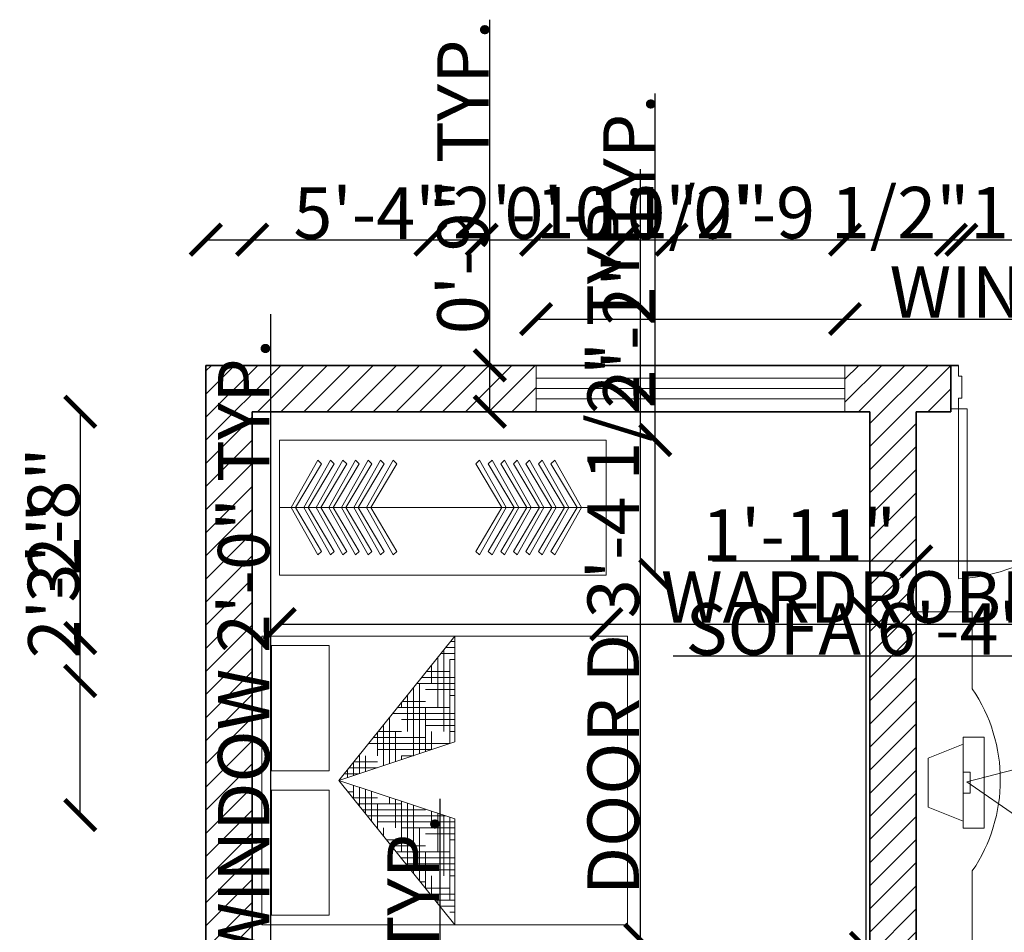
# Model space of a CAD drawing. Units: inches. Extents: x 1957 to 2456, y 1504 to 2088.
# Tile 5 of 6: x 2029 to 2220, y 1911 to 2088. Entities that reach past the tile are written whole.
import ezdxf

# ---------------------------------------------------------------- set-up
doc = ezdxf.new("R2010")
doc.units = ezdxf.units.IN
doc.header["$LTSCALE"] = 2
for name, color, linetype, lineweight in [('A-ANNO-DIMS', 2, 'Continuous', 18), ('A-FURN', 8, 'Continuous', 18), ('A-WALL-PATT', 8, 'Continuous', 13), ('Doors', 42, 'Continuous', 18), ('shelves', 204, 'Continuous', 18), ('Walls', 7, 'Continuous', 35), ('Windows', 140, 'Continuous', 18)]:
    doc.layers.add(name, color=color, linetype=linetype, lineweight=lineweight)
doc.styles.get("Standard").update_dxf_attribs({"font": 'arial.ttf'})
doc.dimstyles.get("Standard").update_dxf_attribs({"dimtxt": 10, "dimasz": 6, "dimexe": 0.18, "dimexo": 0.0625, "dimgap": 0.09, "dimtad": 1, "dimdec": 1, "dimzin": 0, "dimdsep": 46, "dimlunit": 4, "dimtxsty": 'Standard', "dimblk": 'ARCHTICK', "dimcen": 0.09, "dimse1": 1, "dimse2": 1, "dimadec": 0, "dimazin": 0, "dimtfac": 1, "dimtdec": 1, "dimtofl": 0, "dimtmove": 0, "dimatfit": 3, "dimfxl": 1, "dimtolj": 1, "dimtzin": 0, "dimarcsym": 0})

# ---------------------------------------------------------------- blocks, each defined once
blk = doc.blocks.new('banghe81')
for p, q in [((-500, 3000), (0, 3000)), ((-500, 2312.5), (-500, 3000)), ((0, 3000), (0, 0)), ((-606.9, 1930), (-419.4, 1930)), ((-606.9, 1117.5), (-606.9, 1930)), ((-419.4, 1930), (-419.4, 1117.5)), ((-106.9, 1742.5), (-419.4, 1867.5)), ((-924.7, 1843.4), (-449.7, 1516.6)), ((-106.9, 1305), (-106.9, 1742.5)), ((-481.9, 1617.5), (-481.9, 1430)), ((-419.4, 1617.5), (-481.9, 1617.5)), ((-449.7, 1516.6), (-1057.1, 1361)), ((-481.9, 1430), (-419.4, 1430)), ((-419.4, 1180), (-106.9, 1305)), ((-419.4, 1117.5), (-606.9, 1117.5)), ((-500, 0), (-500, 687.5)), ((0, 0), (-500, 0)), ((-500, 0), (-500, 0))]:
    blk.add_line(p, q)
blk.add_arc((695.3, 1500), 1445.3, 145.79454, 214.20546)
blk = doc.blocks.new('*X4')
at = {"color": 0}
for p, q in [((20.25, 14.8125), (20.2772, 14.8125)), ((20.1739, 14.75), (20.2772, 14.75)), ((20.1875, 14.75), (20.1875, 14.7669)), ((20.199, 14.7812), (20.2772, 14.7812)), ((20.25, 14.3194), (20.25, 14.75)), ((20.1236, 14.6875), (20.25, 14.6875)), ((20.125, 14.5), (20.125, 14.6893)), ((20.1487, 14.7188), (20.2772, 14.7188)), ((20.1562, 14.625), (20.1562, 14.7281)), ((20.0938, 14.375), (20.0938, 14.6504)), ((20.0984, 14.6562), (20.125, 14.6562)), ((20.0625, 14.2573), (20.0625, 14.6116)), ((20.125, 14.5938), (20.2772, 14.5938)), ((20.2188, 14.3091), (20.2188, 14.625)), ((20.25, 14.625), (20.2772, 14.625)), ((19.9979, 14.5312), (20.2772, 14.5312)), ((20.023, 14.5625), (20.2772, 14.5625)), ((20.0312, 14.2469), (20.0312, 14.5727)), ((19.9727, 14.5), (20.25, 14.5)), ((20, 14.2366), (20, 14.5)), ((20.1875, 14.2987), (20.1875, 14.5)), ((19.9225, 14.4375), (20, 14.4375)), ((19.9476, 14.4688), (20.125, 14.4688)), ((20.25, 14.4375), (20.2772, 14.4375)), ((19.875, 14.25), (19.875, 14.3785)), ((19.9062, 14.375), (19.9062, 14.4174)), ((19.9688, 14.2262), (19.9688, 14.375)), ((20, 14.375), (20.2772, 14.375)), ((20.125, 14.4062), (20.2772, 14.4062)), ((20.1562, 14.2884), (20.1562, 14.375)), ((19.8438, 14.1848), (19.8438, 14.3397)), ((19.875, 14.3438), (20.2772, 14.3438)), ((19.7967, 14.2812), (20.125, 14.2812)), ((19.8125, 14.1744), (19.8125, 14.3008)), ((19.8219, 14.3125), (20.2291, 14.3125)), ((19.75, 14.1537), (19.75, 14.2231)), ((19.7716, 14.25), (20, 14.25)), ((19.7812, 14.1641), (19.7812, 14.262)), ((19.9375, 14.2159), (19.9375, 14.25)), ((19.7213, 14.1875), (19.75, 14.1875)), ((19.7465, 14.2188), (19.875, 14.2188)), ((19.7018, 14.0938), (19.7786, 14.0938)), ((19.7188, 14.0726), (19.7188, 14.1136)), ((19.75, 14.0338), (19.75, 14.1032)), ((19.7812, 13.9949), (19.7812, 14.0929)), ((19.8125, 14), (19.8125, 14.0825)), ((19.7269, 14.0625), (19.8728, 14.0625)), ((19.752, 14.0312), (19.875, 14.0312)), ((19.9062, 13.8396), (19.9062, 14.0514)), ((19.9375, 13.8007), (19.9375, 14.0411)), ((19.9688, 13.875), (19.9688, 14.0307)), ((20, 14), (20, 14.0204)), ((19.875, 13.8784), (19.875, 14)), ((19.875, 13.9688), (20.1557, 13.9688)), ((20, 14), (20.0614, 14)), ((20.0625, 13.6454), (20.0625, 13.9996)), ((20.0938, 13.625), (20.0938, 13.9893)), ((20.125, 13.75), (20.125, 13.9789)), ((20.1562, 13.875), (20.1562, 13.9686)), ((19.8275, 13.9375), (20.25, 13.9375)), ((20.25, 13.5), (20.25, 13.9375)), ((19.8526, 13.9062), (20.125, 13.9062)), ((19.8777, 13.875), (20, 13.875)), ((20.0312, 13.6842), (20.0312, 13.875)), ((20.2188, 13.4511), (20.2188, 13.875)), ((20.25, 13.875), (20.2772, 13.875)), ((20, 13.8125), (20.2772, 13.8125)), ((20.125, 13.8438), (20.2772, 13.8438)), ((19.9532, 13.7812), (20.2772, 13.7812)), ((19.9783, 13.75), (20.25, 13.75)), ((20, 13.723), (20, 13.75)), ((20.0035, 13.7188), (20.125, 13.7188)), ((20.1875, 13.49), (20.1875, 13.75)), ((20.25, 13.6875), (20.2772, 13.6875)), ((20.0789, 13.625), (20.2772, 13.625)), ((20.125, 13.6562), (20.2772, 13.6562)), ((20.1562, 13.5288), (20.1562, 13.625)), ((20.104, 13.5938), (20.2772, 13.5938)), ((20.1292, 13.5625), (20.25, 13.5625)), ((20.2046, 13.4688), (20.2772, 13.4688)), ((20.25, 13.5), (20.2772, 13.5)), ((20.2297, 13.4375), (20.2772, 13.4375)), ((20.2549, 13.4062), (20.2772, 13.4062))]:
    blk.add_line(p, q, dxfattribs=at)
blk = doc.blocks.new('MAT-P13')
for p, q in [((-0.75, 0), (0.75, 0)), ((-0.75, 0), (-0.75, -1.9)), ((0.75, 0), (0.75, -1.9)), ((-0.7, -0.05), (-0.7, -0.35)), ((-0.7, -0.05), (-0.05, -0.05)), ((-0.05, -0.35), (-0.05, -0.05)), ((0.05, -0.05), (0.7, -0.05)), ((0.05, -0.35), (0.05, -0.05)), ((0.7, -0.05), (0.7, -0.35)), ((-0.7, -0.35), (-0.05, -0.35)), ((0.05, -0.35), (0.7, -0.35)), ((-0.75, -1.0034), (0, -0.4)), ((0, -0.4), (-0.75, -1.0034)), ((0, -0.4), (-0.2, -1.0034)), ((0, -0.4), (0.2, -1.0034)), ((0, -0.4), (0.75, -1.0034)), ((-0.75, -1.0034), (-0.2, -1.0034)), ((0.2, -1.0034), (0.75, -1.0034)), ((0.75, -1.9), (-0.75, -1.9))]:
    blk.add_line(p, q)
at = {"xscale": -1, "rotation": 90}
blk.add_blockref('*X4', (14.1285, 19.2738), dxfattribs=at)
blk = doc.blocks.new('AP0B05')
for p, q in [((35, 100), (35, 880)), ((75, 100), (75, 878.9))]:
    blk.add_line(p, q)
for points in [[(0, 100), (0, -100), (35, -100), (35, -50), (50, -50), (50, 50), (35, 50), (35, 100)], [(850, 100), (850, -100), (815, -100), (815, -50), (800, -50), (800, 50), (815, 50), (815, 100)]]:
    blk.add_lwpolyline(points, close=True)
blk.add_lwpolyline([(35, 100), (75, 100)])
blk.add_arc((-2.4, 62.6), 818.3, 2.6212, 87.3788)
blk = doc.blocks.new('WIN-60IN')
for p, q in [((0, 6.5), (60, 6.5)), ((0, 4.5), (60, 4.5)), ((0, 2.5), (60, 2.5))]:
    blk.add_line(p, q)
blk.add_lwpolyline([(0, 9), (60, 9), (60, 0), (0, 0)], close=True)
blk = doc.blocks.new('WARDROBE-RAIL')
blk.add_line((0, 13.12), (63.46, 13.12))
blk.add_lwpolyline([(0, 26.23), (63.46, 26.23), (63.46, 0), (0, 0)], close=True)
for points in [[(2.25, 13.12), (7.43, 22.31), (8.16, 21.63), (3.1, 13.12)], [(4.68, 13.12), (9.87, 22.31), (10.6, 21.63), (5.54, 13.12)], [(7.12, 13.12), (12.3, 22.31), (13.03, 21.63), (7.98, 13.12)], [(9.56, 13.12), (14.74, 22.31), (15.47, 21.63), (10.41, 13.12)], [(11.99, 13.12), (17.18, 22.31), (17.91, 21.63), (12.85, 13.12)], [(14.43, 13.12), (19.61, 22.31), (20.34, 21.63), (15.29, 13.12)], [(16.87, 13.12), (22.05, 22.31), (22.78, 21.63), (17.72, 13.12)], [(44.01, 13.12), (38.82, 22.31), (38.09, 21.63), (43.15, 13.12)], [(46.44, 13.12), (41.26, 22.31), (40.53, 21.63), (45.59, 13.12)], [(48.88, 13.12), (43.7, 22.31), (42.96, 21.63), (48.02, 13.12)], [(51.31, 13.12), (46.13, 22.31), (45.4, 21.63), (50.46, 13.12)], [(53.75, 13.12), (48.57, 22.31), (47.84, 21.63), (52.89, 13.12)], [(56.19, 13.12), (51.01, 22.31), (50.27, 21.63), (55.33, 13.12)], [(58.62, 13.12), (53.44, 22.31), (52.71, 21.63), (57.77, 13.12)], [(2.25, 13.12), (7.43, 3.92), (8.16, 4.61), (3.1, 13.12)], [(4.68, 13.12), (9.87, 3.92), (10.6, 4.61), (5.54, 13.12)], [(7.12, 13.12), (12.3, 3.92), (13.03, 4.61), (7.98, 13.12)], [(9.56, 13.12), (14.74, 3.92), (15.47, 4.61), (10.41, 13.12)], [(11.99, 13.12), (17.18, 3.92), (17.91, 4.61), (12.85, 13.12)], [(14.43, 13.12), (19.61, 3.92), (20.34, 4.61), (15.29, 13.12)], [(16.87, 13.12), (22.05, 3.92), (22.78, 4.61), (17.72, 13.12)], [(44.01, 13.12), (38.82, 3.92), (38.09, 4.61), (43.15, 13.12)], [(46.44, 13.12), (41.26, 3.92), (40.53, 4.61), (45.59, 13.12)], [(48.88, 13.12), (43.7, 3.92), (42.96, 4.61), (48.02, 13.12)], [(51.31, 13.12), (46.13, 3.92), (45.4, 4.61), (50.46, 13.12)], [(53.75, 13.12), (48.57, 3.92), (47.84, 4.61), (52.89, 13.12)], [(56.19, 13.12), (51.01, 3.92), (50.27, 4.61), (55.33, 13.12)], [(58.62, 13.12), (53.44, 3.92), (52.71, 4.61), (57.77, 13.12)]]:
    blk.add_lwpolyline(points)
blk = doc.blocks.new('_ArchTick')
at = {"color": 0, "linetype": 'ByBlock', "const_width": 0.15}
blk.add_lwpolyline([(-0.5, -0.5), (0.5, 0.5)], dxfattribs=at)
blk = doc.blocks.new('*D17')
at = {"layer": 'A-ANNO-DIMS', "color": 0, "lineweight": -2, "transparency": 16777216}
for p, q in [((2149.43, 1909.65), (2149.43, 2059.35)), ((2149.43, 1869.22), (2149.43, 1909.65))]:
    blk.add_line(p, q, dxfattribs=at)
at = {"layer": 'Defpoints', "color": 0, "transparency": 16777216}
for p in [(2149.43, 1909.65), (2155.49, 1909.65), (2155.49, 1869.22)]:
    blk.add_point(p, dxfattribs=at)
at = {"layer": 'A-ANNO-DIMS', "color": 0, "lineweight": -2, "transparency": 16777216, "xscale": 6, "yscale": 6, "zscale": 6}
for p, rotation in [((2149.43, 1909.65), 90), ((2149.43, 1869.22), 270)]:
    blk.add_blockref('_ArchTick', p, dxfattribs=dict(at, rotation=rotation))
at = {"layer": 'A-ANNO-DIMS', "color": 0, "transparency": 16777216, "insert": (2144.16, 1987.5), "char_height": 10, "attachment_point": 5, "rotation": 90}
blk.add_mtext('\\A1;DOOR D 3\'-4 1/2" TYP.', dxfattribs=at)
blk = doc.blocks.new('*D21')
at = {"layer": 'A-ANNO-DIMS', "color": 0, "lineweight": -2, "transparency": 16777216}
for p, q in [((2110.57, 1795.08), (2110.57, 1937.02)), ((2110.57, 1760.22), (2110.57, 1795.08))]:
    blk.add_line(p, q, dxfattribs=at)
at = {"layer": 'Defpoints', "color": 0, "transparency": 16777216}
for p in [(2110.57, 1795.08), (2115.8, 1795.08), (2115.8, 1760.22)]:
    blk.add_point(p, dxfattribs=at)
at = {"layer": 'A-ANNO-DIMS', "color": 0, "lineweight": -2, "transparency": 16777216, "xscale": 6, "yscale": 6, "zscale": 6}
for p, rotation in [((2110.57, 1795.08), 90), ((2110.57, 1760.22), 270)]:
    blk.add_blockref('_ArchTick', p, dxfattribs=dict(at, rotation=rotation))
at = {"layer": 'A-ANNO-DIMS', "color": 0, "transparency": 16777216, "insert": (2105.3, 1869.05), "char_height": 10, "attachment_point": 5, "rotation": 90}
blk.add_mtext('\\A1;DOOR D1 2\'-11" TYP.', dxfattribs=at)
blk = doc.blocks.new('*D25')
at = {"layer": 'A-ANNO-DIMS', "color": 0, "lineweight": -2, "transparency": 16777216}
for p, q in [((2129.18, 2030.22), (2189.18, 2030.22)), ((2189.18, 2030.22), (2321.9, 2030.22))]:
    blk.add_line(p, q, dxfattribs=at)
at = {"layer": 'Defpoints', "color": 0, "transparency": 16777216}
for p in [(2189.18, 2030.22), (2129.18, 2021.22), (2189.18, 2021.22)]:
    blk.add_point(p, dxfattribs=at)
at = {"layer": 'A-ANNO-DIMS', "color": 0, "lineweight": -2, "transparency": 16777216, "xscale": 6, "yscale": 6, "zscale": 6, "rotation": 180}
blk.add_blockref('_ArchTick', (2129.18, 2030.22), dxfattribs=at)
at = {"layer": 'A-ANNO-DIMS', "color": 0, "lineweight": -2, "transparency": 16777216, "xscale": 6, "yscale": 6, "zscale": 6}
blk.add_blockref('_ArchTick', (2189.18, 2030.22), dxfattribs=at)
at = {"layer": 'A-ANNO-DIMS', "color": 0, "transparency": 16777216, "insert": (2258.54, 2035.48), "char_height": 10, "attachment_point": 5}
blk.add_mtext('\\A1;WINDOW 5\'-0" TYP.', dxfattribs=at)
blk = doc.blocks.new('*D26')
at = {"layer": 'A-ANNO-DIMS', "color": 0, "lineweight": -2, "transparency": 16777216}
for p, q in [((2120.18, 2021.22), (2120.18, 2088.35)), ((2120.18, 2012.22), (2120.18, 2021.22))]:
    blk.add_line(p, q, dxfattribs=at)
at = {"layer": 'Defpoints', "color": 0, "transparency": 16777216}
for p in [(2120.18, 2021.22), (2129.18, 2021.22), (2129.18, 2012.22)]:
    blk.add_point(p, dxfattribs=at)
at = {"layer": 'A-ANNO-DIMS', "color": 0, "lineweight": -2, "transparency": 16777216, "xscale": 6, "yscale": 6, "zscale": 6}
for p, rotation in [((2120.18, 2021.22), 90), ((2120.18, 2012.22), 270)]:
    blk.add_blockref('_ArchTick', p, dxfattribs=dict(at, rotation=rotation))
at = {"layer": 'A-ANNO-DIMS', "color": 0, "transparency": 16777216, "insert": (2114.98, 2057.79), "char_height": 10, "attachment_point": 5, "rotation": 90}
blk.add_mtext('\\A1;0\'-9" TYP.', dxfattribs=at)
blk = doc.blocks.new('*D27')
at = {"layer": 'A-ANNO-DIMS', "color": 0, "lineweight": -2, "transparency": 16777216}
for p, q in [((2077.63, 1857.22), (2077.63, 2031.19)), ((2077.63, 1833.22), (2077.63, 1857.22))]:
    blk.add_line(p, q, dxfattribs=at)
at = {"layer": 'Defpoints', "color": 0, "transparency": 16777216}
for p in [(2074.03, 1857.22), (2077.63, 1857.22), (2074.03, 1833.22)]:
    blk.add_point(p, dxfattribs=at)
at = {"layer": 'A-ANNO-DIMS', "color": 0, "lineweight": -2, "transparency": 16777216, "xscale": 6, "yscale": 6, "zscale": 6}
for p, rotation in [((2077.63, 1857.22), 90), ((2077.63, 1833.22), 270)]:
    blk.add_blockref('_ArchTick', p, dxfattribs=dict(at, rotation=rotation))
at = {"layer": 'A-ANNO-DIMS', "color": 0, "transparency": 16777216, "insert": (2072.37, 1947.2), "char_height": 10, "attachment_point": 5, "rotation": 90}
blk.add_mtext('\\A1;VENT WINDOW 2\'-0" TYP.', dxfattribs=at)
blk = doc.blocks.new('*D31')
at = {"layer": 'A-ANNO-DIMS', "color": 0, "lineweight": -2, "transparency": 16777216}
for p, q in [((2079.36, 1970.96), (2142.81, 1970.96)), ((2142.81, 1970.96), (2319.81, 1970.96))]:
    blk.add_line(p, q, dxfattribs=at)
at = {"layer": 'Defpoints', "color": 0, "transparency": 16777216}
for p in [(2079.36, 1980.47), (2142.81, 1980.47), (2142.81, 1970.96)]:
    blk.add_point(p, dxfattribs=at)
at = {"layer": 'A-ANNO-DIMS', "color": 0, "lineweight": -2, "transparency": 16777216, "xscale": 6, "yscale": 6, "zscale": 6, "rotation": 180}
blk.add_blockref('_ArchTick', (2079.36, 1970.96), dxfattribs=at)
at = {"layer": 'A-ANNO-DIMS', "color": 0, "lineweight": -2, "transparency": 16777216, "xscale": 6, "yscale": 6, "zscale": 6}
blk.add_blockref('_ArchTick', (2142.81, 1970.96), dxfattribs=at)
at = {"layer": 'A-ANNO-DIMS', "color": 0, "transparency": 16777216, "insert": (2234.31, 1976.22), "char_height": 10, "attachment_point": 5}
blk.add_mtext('\\A1;WARDROBE 5\'-3 1/2" TYP.', dxfattribs=at)
blk = doc.blocks.new('*D32')
at = {"layer": 'A-ANNO-DIMS', "color": 0, "lineweight": -2, "transparency": 16777216}
for p, q in [((2152.33, 2006.71), (2152.33, 2074.01)), ((2152.33, 1980.47), (2152.33, 2006.71))]:
    blk.add_line(p, q, dxfattribs=at)
at = {"layer": 'Defpoints', "color": 0, "transparency": 16777216}
for p in [(2142.81, 2006.71), (2152.33, 2006.71), (2142.81, 1980.47)]:
    blk.add_point(p, dxfattribs=at)
at = {"layer": 'A-ANNO-DIMS', "color": 0, "lineweight": -2, "transparency": 16777216, "xscale": 6, "yscale": 6, "zscale": 6}
for p, rotation in [((2152.33, 2006.71), 90), ((2152.33, 1980.47), 270)]:
    blk.add_blockref('_ArchTick', p, dxfattribs=dict(at, rotation=rotation))
at = {"layer": 'A-ANNO-DIMS', "color": 0, "transparency": 16777216, "insert": (2147.22, 2043.36), "char_height": 10, "attachment_point": 5, "rotation": 90}
blk.add_mtext('\\A1;2\'-2" TYP.', dxfattribs=at)
blk = doc.blocks.new('*D35')
at = {"layer": 'A-ANNO-DIMS', "color": 0, "lineweight": -2, "transparency": 16777216}
for p, q in [((2264.8, 1964.77), (2155.8, 1964.77)), ((2340.57, 1964.77), (2264.8, 1964.77))]:
    blk.add_line(p, q, dxfattribs=at)
at = {"layer": 'Defpoints', "color": 0, "transparency": 16777216}
for p in [(2264.8, 1976.14), (2340.57, 1976.14), (2264.8, 1964.77)]:
    blk.add_point(p, dxfattribs=at)
at = {"layer": 'A-ANNO-DIMS', "color": 0, "lineweight": -2, "transparency": 16777216, "xscale": 6, "yscale": 6, "zscale": 6, "rotation": 180}
blk.add_blockref('_ArchTick', (2264.8, 1964.77), dxfattribs=at)
at = {"layer": 'A-ANNO-DIMS', "color": 0, "lineweight": -2, "transparency": 16777216, "xscale": 6, "yscale": 6, "zscale": 6}
blk.add_blockref('_ArchTick', (2340.57, 1964.77), dxfattribs=at)
at = {"layer": 'A-ANNO-DIMS', "color": 0, "transparency": 16777216, "insert": (2207.3, 1970.03), "char_height": 10, "attachment_point": 5}
blk.add_mtext('\\A1;SOFA 6\'-4" TYP.', dxfattribs=at)
blk = doc.blocks.new('*D39')
at = {"layer": 'A-ANNO-DIMS', "color": 0, "lineweight": -2, "transparency": 16777216}
for p, q in [((2193.24, 1973.36), (2193.24, 1908.07)), ((2193.24, 1908.07), (2193.24, 1757.83))]:
    blk.add_line(p, q, dxfattribs=at)
at = {"layer": 'Defpoints', "color": 0, "transparency": 16777216}
for p in [(2203.03, 1973.36), (2193.24, 1908.07), (2203.03, 1908.07)]:
    blk.add_point(p, dxfattribs=at)
at = {"layer": 'A-ANNO-DIMS', "color": 0, "lineweight": -2, "transparency": 16777216, "xscale": 6, "yscale": 6, "zscale": 6}
for p, rotation in [((2193.24, 1973.36), 90), ((2193.24, 1908.07), 270)]:
    blk.add_blockref('_ArchTick', p, dxfattribs=dict(at, rotation=rotation))
at = {"layer": 'A-ANNO-DIMS', "color": 0, "transparency": 16777216, "insert": (2187.98, 1829.95), "char_height": 10, "attachment_point": 5, "rotation": 90}
blk.add_mtext('\\A1;TV CONSOLE 5\'-5 1/2"', dxfattribs=at)
blk = doc.blocks.new('*D40')
at = {"layer": 'A-ANNO-DIMS', "color": 0, "lineweight": -2, "transparency": 16777216}
for p, q in [((2203.03, 1983.16), (2163.44, 1983.16)), ((2226.04, 1983.16), (2203.03, 1983.16))]:
    blk.add_line(p, q, dxfattribs=at)
at = {"layer": 'Defpoints', "color": 0, "transparency": 16777216}
for p in [(2203.03, 1983.16), (2203.03, 1973.36), (2226.04, 1973.36)]:
    blk.add_point(p, dxfattribs=at)
at = {"layer": 'A-ANNO-DIMS', "color": 0, "lineweight": -2, "transparency": 16777216, "xscale": 6, "yscale": 6, "zscale": 6, "rotation": 180}
blk.add_blockref('_ArchTick', (2203.03, 1983.16), dxfattribs=at)
at = {"layer": 'A-ANNO-DIMS', "color": 0, "lineweight": -2, "transparency": 16777216, "xscale": 6, "yscale": 6, "zscale": 6}
blk.add_blockref('_ArchTick', (2226.04, 1983.16), dxfattribs=at)
at = {"layer": 'A-ANNO-DIMS', "color": 0, "transparency": 16777216, "insert": (2180.24, 1988.27), "char_height": 10, "attachment_point": 5}
blk.add_mtext('\\A1;1\'-11"', dxfattribs=at)
blk = doc.blocks.new('*D47')
at = {"layer": 'A-ANNO-DIMS', "color": 0, "lineweight": -2, "transparency": 16777216}
blk.add_line((2065.03, 2045.62), (2129.18, 2045.62), dxfattribs=at)
at = {"layer": 'Defpoints', "color": 0, "transparency": 16777216}
for p in [(2129.18, 2045.62), (2065.03, 2021.22), (2129.18, 2021.22)]:
    blk.add_point(p, dxfattribs=at)
at = {"layer": 'A-ANNO-DIMS', "color": 0, "lineweight": -2, "transparency": 16777216, "xscale": 6, "yscale": 6, "zscale": 6, "rotation": 180}
blk.add_blockref('_ArchTick', (2065.03, 2045.62), dxfattribs=at)
at = {"layer": 'A-ANNO-DIMS', "color": 0, "lineweight": -2, "transparency": 16777216, "xscale": 6, "yscale": 6, "zscale": 6}
blk.add_blockref('_ArchTick', (2129.18, 2045.62), dxfattribs=at)
at = {"layer": 'A-ANNO-DIMS', "color": 0, "transparency": 16777216, "insert": (2097.1, 2050.79), "char_height": 10, "attachment_point": 5}
blk.add_mtext('\\A1;5\'-4"', dxfattribs=at)
blk = doc.blocks.new('*D48')
at = {"layer": 'A-ANNO-DIMS', "color": 0, "lineweight": -2, "transparency": 16777216}
for p, q in [((2189.18, 2045.62), (2209.75, 2045.62)), ((2209.75, 2045.62), (2264.87, 2045.62))]:
    blk.add_line(p, q, dxfattribs=at)
at = {"layer": 'Defpoints', "color": 0, "transparency": 16777216}
for p in [(2209.75, 2045.62), (2189.18, 2021.22), (2209.75, 2021.22)]:
    blk.add_point(p, dxfattribs=at)
at = {"layer": 'A-ANNO-DIMS', "color": 0, "lineweight": -2, "transparency": 16777216, "xscale": 6, "yscale": 6, "zscale": 6, "rotation": 180}
blk.add_blockref('_ArchTick', (2189.18, 2045.62), dxfattribs=at)
at = {"layer": 'A-ANNO-DIMS', "color": 0, "lineweight": -2, "transparency": 16777216, "xscale": 6, "yscale": 6, "zscale": 6}
blk.add_blockref('_ArchTick', (2209.75, 2045.62), dxfattribs=at)
at = {"layer": 'A-ANNO-DIMS', "color": 0, "transparency": 16777216, "insert": (2240.31, 2050.88), "char_height": 10, "attachment_point": 5}
blk.add_mtext('\\A1;1\'-8 1/2"', dxfattribs=at)
blk = doc.blocks.new('*D50')
at = {"layer": 'A-ANNO-DIMS', "color": 0, "lineweight": -2, "transparency": 16777216}
blk.add_line((2040.63, 2012.22), (2040.63, 1968.25), dxfattribs=at)
at = {"layer": 'Defpoints', "color": 0, "transparency": 16777216}
for p in [(2362.03, 2012.22), (2040.63, 1968.25), (2362.03, 1968.25)]:
    blk.add_point(p, dxfattribs=at)
at = {"layer": 'A-ANNO-DIMS', "color": 0, "lineweight": -2, "transparency": 16777216, "xscale": 6, "yscale": 6, "zscale": 6}
for p, rotation in [((2040.63, 2012.22), 90), ((2040.63, 1968.25), 270)]:
    blk.add_blockref('_ArchTick', p, dxfattribs=dict(at, rotation=rotation))
at = {"layer": 'A-ANNO-DIMS', "color": 0, "transparency": 16777216, "insert": (2035.43, 1990.23), "char_height": 10, "attachment_point": 5, "rotation": 90}
blk.add_mtext('\\A1;3\'-8"', dxfattribs=at)
blk = doc.blocks.new('*D61')
at = {"layer": 'A-ANNO-DIMS', "color": 0, "lineweight": -2, "transparency": 16777216}
for p, q in [((2211.8, 2045.62), (2247.38, 2045.62)), ((2247.38, 2045.62), (2311.38, 2045.62))]:
    blk.add_line(p, q, dxfattribs=at)
at = {"layer": 'Defpoints', "color": 0, "transparency": 16777216}
for p in [(2247.38, 2045.62), (2211.8, 1820.22), (2247.38, 1820.22)]:
    blk.add_point(p, dxfattribs=at)
at = {"layer": 'A-ANNO-DIMS', "color": 0, "lineweight": -2, "transparency": 16777216, "xscale": 6, "yscale": 6, "zscale": 6, "rotation": 180}
blk.add_blockref('_ArchTick', (2211.8, 2045.62), dxfattribs=at)
at = {"layer": 'A-ANNO-DIMS', "color": 0, "lineweight": -2, "transparency": 16777216, "xscale": 6, "yscale": 6, "zscale": 6}
blk.add_blockref('_ArchTick', (2247.38, 2045.62), dxfattribs=at)
at = {"layer": 'A-ANNO-DIMS', "color": 0, "transparency": 16777216, "insert": (2282.38, 2050.88), "char_height": 10, "attachment_point": 5}
blk.add_mtext('\\A1;2\'-11 1/2"', dxfattribs=at)
blk = doc.blocks.new('*D62')
at = {"layer": 'A-ANNO-DIMS', "color": 0, "lineweight": -2, "transparency": 16777216}
for p, q in [((2074.03, 2045.62), (2108.63, 2045.62)), ((2108.63, 2045.62), (2172.63, 2045.62))]:
    blk.add_line(p, q, dxfattribs=at)
at = {"layer": 'Defpoints', "color": 0, "transparency": 16777216}
for p in [(2108.63, 2045.62), (2074.03, 1547.22), (2108.63, 1547.22)]:
    blk.add_point(p, dxfattribs=at)
at = {"layer": 'A-ANNO-DIMS', "color": 0, "lineweight": -2, "transparency": 16777216, "xscale": 6, "yscale": 6, "zscale": 6, "rotation": 180}
blk.add_blockref('_ArchTick', (2074.03, 2045.62), dxfattribs=at)
at = {"layer": 'A-ANNO-DIMS', "color": 0, "lineweight": -2, "transparency": 16777216, "xscale": 6, "yscale": 6, "zscale": 6}
blk.add_blockref('_ArchTick', (2108.63, 2045.62), dxfattribs=at)
at = {"layer": 'A-ANNO-DIMS', "color": 0, "transparency": 16777216, "insert": (2143.63, 2050.88), "char_height": 10, "attachment_point": 5}
blk.add_mtext('\\A1;2\'-10 1/2"', dxfattribs=at)
blk = doc.blocks.new('*D63')
at = {"layer": 'A-ANNO-DIMS', "color": 0, "lineweight": -2, "transparency": 16777216}
for p, q in [((2108.63, 2045.62), (2118.63, 2045.62)), ((2118.63, 2045.62), (2159.16, 2045.62))]:
    blk.add_line(p, q, dxfattribs=at)
at = {"layer": 'Defpoints', "color": 0, "transparency": 16777216}
for p in [(2118.63, 2045.62), (2108.63, 1547.22), (2118.63, 1547.22)]:
    blk.add_point(p, dxfattribs=at)
at = {"layer": 'A-ANNO-DIMS', "color": 0, "lineweight": -2, "transparency": 16777216, "xscale": 6, "yscale": 6, "zscale": 6, "rotation": 180}
blk.add_blockref('_ArchTick', (2108.63, 2045.62), dxfattribs=at)
at = {"layer": 'A-ANNO-DIMS', "color": 0, "lineweight": -2, "transparency": 16777216, "xscale": 6, "yscale": 6, "zscale": 6}
blk.add_blockref('_ArchTick', (2118.63, 2045.62), dxfattribs=at)
at = {"layer": 'A-ANNO-DIMS', "color": 0, "transparency": 16777216, "insert": (2141.89, 2050.81), "char_height": 10, "attachment_point": 5}
blk.add_mtext('\\A1;0\'-10"', dxfattribs=at)
blk = doc.blocks.new('*D65')
at = {"layer": 'A-ANNO-DIMS', "color": 0, "lineweight": -2, "transparency": 16777216}
for p, q in [((2040.63, 1959.92), (2040.63, 1992.85)), ((2040.63, 1933.88), (2040.63, 1959.92))]:
    blk.add_line(p, q, dxfattribs=at)
at = {"layer": 'Defpoints', "color": 0, "transparency": 16777216}
for p in [(2040.63, 1959.92), (2290.6, 1959.92), (2290.6, 1933.88)]:
    blk.add_point(p, dxfattribs=at)
at = {"layer": 'A-ANNO-DIMS', "color": 0, "lineweight": -2, "transparency": 16777216, "xscale": 6, "yscale": 6, "zscale": 6}
for p, rotation in [((2040.63, 1959.92), 90), ((2040.63, 1933.88), 270)]:
    blk.add_blockref('_ArchTick', p, dxfattribs=dict(at, rotation=rotation))
at = {"layer": 'A-ANNO-DIMS', "color": 0, "transparency": 16777216, "insert": (2035.52, 1979.39), "char_height": 10, "attachment_point": 5, "rotation": 90}
blk.add_mtext('\\A1;2\'-2"', dxfattribs=at)
blk = doc.blocks.new('*D69')
at = {"layer": 'A-ANNO-DIMS', "color": 0, "lineweight": -2, "transparency": 16777216}
for p, q in [((2146.03, 2045.62), (2155.49, 2045.62)), ((2155.49, 2045.62), (2211.56, 2045.62))]:
    blk.add_line(p, q, dxfattribs=at)
at = {"layer": 'Defpoints', "color": 0, "transparency": 16777216}
for p in [(2155.49, 2045.62), (2146.03, 1878.22), (2155.49, 1878.22)]:
    blk.add_point(p, dxfattribs=at)
at = {"layer": 'A-ANNO-DIMS', "color": 0, "lineweight": -2, "transparency": 16777216, "xscale": 6, "yscale": 6, "zscale": 6, "rotation": 180}
blk.add_blockref('_ArchTick', (2146.03, 2045.62), dxfattribs=at)
at = {"layer": 'A-ANNO-DIMS', "color": 0, "lineweight": -2, "transparency": 16777216, "xscale": 6, "yscale": 6, "zscale": 6}
blk.add_blockref('_ArchTick', (2155.49, 2045.62), dxfattribs=at)
at = {"layer": 'A-ANNO-DIMS', "color": 0, "transparency": 16777216, "insert": (2186.53, 2050.88), "char_height": 10, "attachment_point": 5}
blk.add_mtext('\\A1;0\'-9 1/2"', dxfattribs=at)

msp = doc.modelspace()

# ---------------------------------------------------------------- hatches: boundary and pattern name
at = {"layer": 'A-WALL-PATT', "transparency": 33554585}
h = msp.add_hatch(dxfattribs=at)
h.set_pattern_fill('ANSI31', color=256)
h.paths.add_polyline_path([(2129.18, 2021.22), (2065.03, 2021.22), (2065.03, 1857.22), (2074.03, 1857.22), (2074.03, 1869.22), (2115.8, 1869.22), (2115.8, 1878.22), (2074.03, 1878.22), (2074.03, 2012.22), (2129.18, 2012.22)])
h.paths.add_polyline_path([(2209.75, 2021.22), (2189.18, 2021.22), (2189.18, 2012.22), (2194.03, 2012.22), (2194.03, 1878.22), (2190.56, 1878.22), (2190.56, 1869.22), (2203.03, 1869.22), (2203.03, 2012.22), (2209.75, 2012.22)])
h.paths.add_polyline_path([(2273.18, 2021.22), (2245.68, 2021.22), (2245.68, 2012.22), (2273.18, 2012.22)])
h.paths.add_polyline_path([(2371.03, 2021.22), (2333.18, 2021.22), (2333.18, 2012.22), (2362.03, 2012.22), (2362.03, 1968.25), (2371.03, 1968.25)])
h.paths.add_polyline_path([(2371.03, 1869.22), (2367.03, 1869.22), (2367.03, 1546.41), (2371.03, 1546.41)])
h.paths.add_polyline_path([(2317.03, 1820.22), (2247.38, 1820.22), (2247.38, 1811.22), (2308.03, 1811.22), (2308.03, 1697.22), (2284.03, 1697.22), (2284.03, 1688.22), (2317.03, 1688.22)])
h.paths.add_polyline_path([(2236.03, 1697.22), (2203.03, 1697.22), (2203.03, 1811.22), (2211.8, 1811.22), (2211.8, 1820.22), (2194.03, 1820.22), (2194.03, 1619.22), (2074.03, 1619.22), (2074.03, 1610.22), (2203.03, 1610.22), (2203.03, 1688.22), (2236.03, 1688.22)])
h.paths.add_polyline_path([(2153.03, 1869.22), (2155.49, 1869.22), (2155.49, 1877.47), (2155.49, 1878.22), (2146.03, 1878.22), (2146.03, 1871.1), (2146.03, 1869.22), (2149.03, 1869.22), (2149.03, 1821.22), (2074.03, 1821.22), (2074.03, 1833.22), (2065.03, 1833.22), (2065.03, 1805.22), (2074.03, 1805.22), (2074.03, 1817.22), (2149.03, 1817.22), (2149.03, 1769.22), (2146.03, 1769.22), (2146.03, 1760.22), (2153.03, 1760.22), (2156.02, 1760.22), (2156.02, 1760.87), (2156.02, 1769.11), (2153.03, 1769.11)])
h.paths.add_polyline_path([(2074.03, 1781.22), (2065.03, 1781.22), (2065.03, 1758.05), (2074.03, 1758.05), (2074.03, 1760.22), (2115.8, 1760.22), (2115.8, 1767.33), (2115.8, 1769.22), (2074.03, 1769.22)])

# ---------------------------------------------------------------- linework, layer by layer
at = {"layer": 'Walls'}
for p, q in [((2065.03, 2021.22), (2065.03, 1538.22)), ((2211.23, 2021.22), (2065.03, 2021.22)), ((2209.75, 2021.22), (2209.75, 2012.22)), ((2074.03, 2012.22), (2074.03, 1878.22)), ((2194.03, 2012.22), (2074.03, 2012.22)), ((2194.03, 2012.22), (2194.03, 1878.22)), ((2203.03, 2012.22), (2203.03, 1869.22)), ((2209.75, 2012.22), (2203.03, 2012.22))]:
    msp.add_line(p, q, dxfattribs=at)

# ---------------------------------------------------------------- block references
at = {"layer": 'A-FURN'}
for name, p, xscale, yscale, zscale, rotation in [('banghe81', (2203.03, 1973.36), 0.0217636098217213, 0.0217636098217213, 0.0217636098217213, 180), ('MAT-P13', (2075.9, 1940.61), 37.39052698416379, 37.39052698416379, 37.39052698416379, 90)]:
    msp.add_blockref(name, p, dxfattribs=dict(at, xscale=xscale, yscale=yscale, zscale=zscale, rotation=rotation))
at = {"layer": 'Doors', "xscale": -0.042270002124437, "yscale": 0.042270002124437, "zscale": 0.042270002124437, "rotation": 180}
msp.add_blockref('AP0B05', (2209.75, 2016.99), dxfattribs=at)
at = {"layer": 'shelves'}
msp.add_blockref('WARDROBE-RAIL', (2079.36, 1980.47), dxfattribs=at)
at = {"layer": 'Windows'}
msp.add_blockref('WIN-60IN', (2129.18, 2012.22), dxfattribs=at)

# ---------------------------------------------------------------- dimensions: what is measured, and where the dimension line sits
at = {"layer": 'A-ANNO-DIMS'}
for base, p1, p2, angle, text, picture, middle in [((2120.18, 2021.22), (2129.18, 2012.22), (2129.18, 2021.22), 90, '<> TYP.', '*D26', (2114.98, 2057.79)), ((2152.33, 2006.71), (2142.81, 1980.47), (2142.81, 2006.71), 90, '<> TYP.', '*D32', (2147.22, 2043.36)), ((2149.43, 1909.65), (2155.49, 1869.22), (2155.49, 1909.65), 90, 'DOOR D <> TYP.', '*D17', (2144.16, 1987.5)), ((2077.63, 1857.22), (2074.03, 1833.22), (2074.03, 1857.22), 90, 'VENT WINDOW <> TYP.', '*D27', (2072.37, 1947.2)), ((2264.8, 1964.77), (2340.57, 1976.14), (2264.8, 1976.14), 180, 'SOFA <> TYP.', '*D35', (2207.3, 1970.03)), ((2193.24, 1908.07), (2203.03, 1973.36), (2203.03, 1908.07), 270, 'TV CONSOLE <>', '*D39', (2187.98, 1829.95)), ((2110.57, 1795.08), (2115.8, 1760.22), (2115.8, 1795.08), 90, 'DOOR D1 <> TYP.', '*D21', (2105.3, 1869.05))]:
    dim = msp.add_linear_dim(base=base, p1=p1, p2=p2, angle=angle, text=text, dimstyle='Standard', override={"dimdec": 1, "dimlfac": 1, "dimrnd": 0, "dimzin": 1, "dimdsep": 46, "dimlunit": 4, "dimfrac": 2}, dxfattribs=at)
    dim.commit()
    dim.dimension.update_dxf_attribs({"geometry": picture, "text_midpoint": middle})
for base, p1, p2, picture, middle in [((2108.63, 2045.62), (2074.03, 1547.22), (2108.63, 1547.22), '*D62', (2143.63, 2050.88)), ((2155.49, 2045.62), (2146.03, 1878.22), (2155.49, 1878.22), '*D69', (2186.53, 2050.88)), ((2209.75, 2045.62), (2189.18, 2021.22), (2209.75, 2021.22), '*D48', (2240.31, 2050.88)), ((2247.38, 2045.62), (2211.8, 1820.22), (2247.38, 1820.22), '*D61', (2282.38, 2050.88)), ((2129.1758, 2045.6189), (2065.0339, 2021.2189), (2129.1758, 2021.2189), '*D47', (2097.1049, 2050.7942)), ((2118.63, 2045.62), (2108.63, 1547.22), (2118.63, 1547.22), '*D63', (2141.89, 2050.81))]:
    dim = msp.add_linear_dim(base=base, p1=p1, p2=p2, dimstyle='Standard', override={"dimdec": 1, "dimlfac": 1, "dimrnd": 0, "dimzin": 1, "dimdsep": 46, "dimlunit": 4, "dimfrac": 2}, dxfattribs=at)
    dim.commit()
    dim.dimension.update_dxf_attribs({"geometry": picture, "text_midpoint": middle})
for base, p1, p2, text, picture, middle in [((2189.18, 2030.22), (2129.18, 2021.22), (2189.18, 2021.22), 'WINDOW <> TYP.', '*D25', (2258.54, 2035.48)), ((2142.8119, 1970.9563), (2079.3559, 1980.4747), (2142.8119, 1980.4747), 'WARDROBE <> TYP.', '*D31', (2234.3112, 1976.2236))]:
    dim = msp.add_linear_dim(base=base, p1=p1, p2=p2, text=text, dimstyle='Standard', override={"dimdec": 1, "dimlfac": 1, "dimrnd": 0, "dimzin": 1, "dimdsep": 46, "dimlunit": 4, "dimfrac": 2}, dxfattribs=at)
    dim.commit()
    dim.dimension.update_dxf_attribs({"geometry": picture, "text_midpoint": middle})
for base, p1, p2, angle, picture, middle in [((2040.63, 1968.25), (2362.03, 2012.22), (2362.03, 1968.25), 90, '*D50', (2035.43, 1990.23)), ((2203.03, 1983.16), (2226.04, 1973.36), (2203.03, 1973.36), 180, '*D40', (2180.24, 1988.27)), ((2040.63, 1959.92), (2290.6, 1933.88), (2290.6, 1959.92), 90, '*D65', (2035.52, 1979.39))]:
    dim = msp.add_linear_dim(base=base, p1=p1, p2=p2, angle=angle, dimstyle='Standard', override={"dimdec": 1, "dimlfac": 1, "dimrnd": 0, "dimzin": 1, "dimdsep": 46, "dimlunit": 4, "dimfrac": 2}, dxfattribs=at)
    dim.commit()
    dim.dimension.update_dxf_attribs({"geometry": picture, "text_midpoint": middle})

doc.saveas('drawing.dxf')
